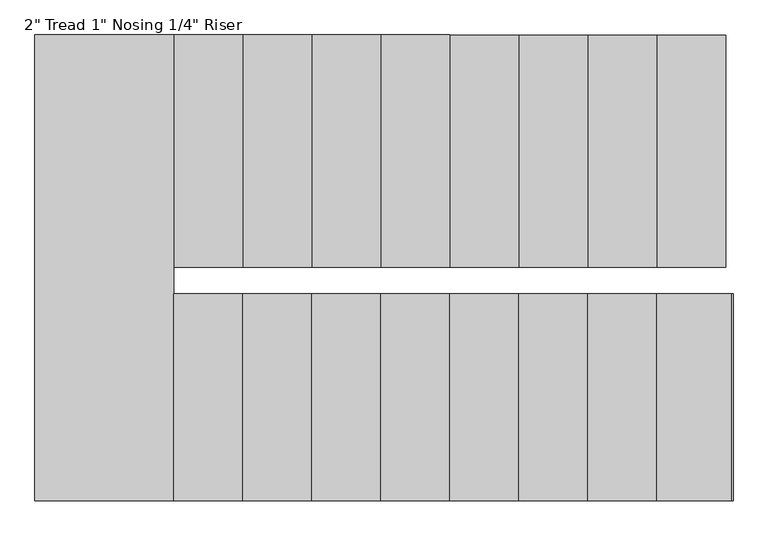
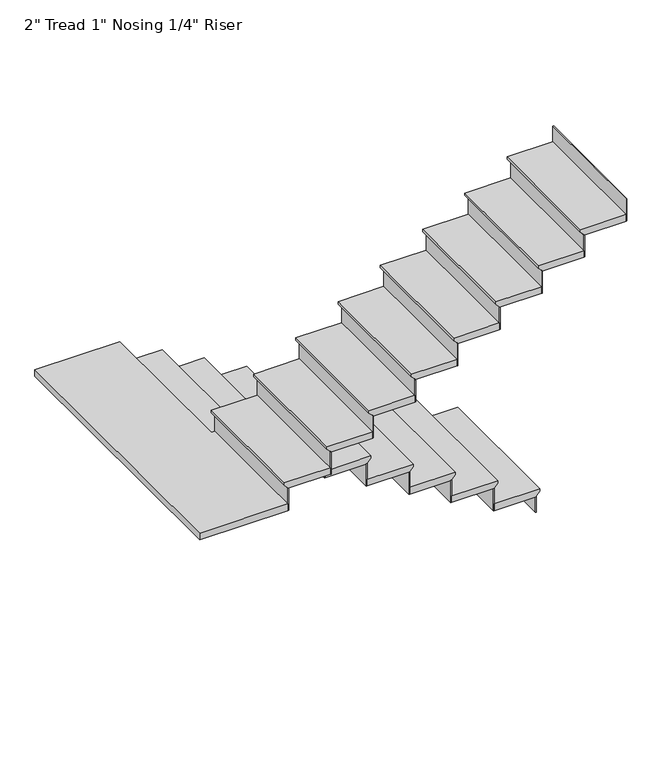
"""IFC4 building model written with IfcOpenShell, lengths in millimetres: stair flight geometry."""

from ifc_helpers import new_model, si_unit, origin, place, context, project, spatial, faceted_brep, source, transform, mapped, element, save


def stair_flight_dc0a5270(model_context):
    return source(origin(), model_context, "Body", "Brep", [
        faceted_brep([(4295.1355783, 9969.5, 150.2833333), (4295.1355783, 9969.5, 169.3333333), (4295.1355783, 8944.6068332, 169.3333333), (4295.1355783, 8944.6068332, 150.2833333), (4269.7355783, 9969.5, 124.8833333), (4269.7355783, 8944.6068332, 124.8833333), (3964.9355783, 9969.5, 169.3333333), (3964.9355783, 8944.6068332, 169.3333333), (4269.7355783, 8944.6068332, 118.5333333), (3964.9355783, 8944.6068332, 118.5333333), (3964.9355783, 9969.5, 118.5333333), (4269.7355783, 9969.5, 118.5333333)], [[[0, 1, 2, 3]], [[4, 0, 3, 5]], [[2, 1, 6, 7]], [[8, 9, 10, 11]], [[2, 7, 9, 8, 5, 3]], [[8, 11, 4, 5]], [[6, 1, 0, 4, 11, 10]], [[7, 6, 10, 9]]]),
        faceted_brep([(4269.7355783, 9969.5, 118.5333333), (4269.7355783, 9969.5, 0.0), (4263.3855783, 9969.5, 0.0), (4263.3855783, 9969.5, 118.5333333), (4269.7355783, 8944.6068332, 118.5333333), (4263.3855783, 8944.6068332, 118.5333333), (4263.3855783, 8944.6068332, 0.0), (4269.7355783, 8944.6068332, 0.0)], [[[0, 1, 2, 3]], [[4, 5, 6, 7]], [[1, 0, 4, 7]], [[2, 1, 7, 6]], [[3, 2, 6, 5]], [[0, 3, 5, 4]]]),
        faceted_brep([(3964.9355783, 9969.5, 287.8666667), (3964.9355783, 9969.5, 118.5333333), (3958.5855783, 9969.5, 118.5333333), (3958.5855783, 9969.5, 287.8666667), (3964.9355783, 8944.6068332, 287.8666667), (3958.5855783, 8944.6068332, 287.8666667), (3958.5855783, 8944.6068332, 118.5333333), (3964.9355783, 8944.6068332, 118.5333333)], [[[0, 1, 2, 3]], [[4, 5, 6, 7]], [[1, 0, 4, 7]], [[2, 1, 7, 6]], [[3, 2, 6, 5]], [[0, 3, 5, 4]]]),
        faceted_brep([(3990.3355783, 8944.6068332, 338.6666667), (3990.3355783, 9969.5, 338.6666667), (3660.1355783, 9969.5, 338.6666667), (3660.1355783, 8944.6068332, 338.6666667), (3964.9355783, 8944.6068332, 287.8666667), (3660.1355783, 8944.6068332, 287.8666667), (3660.1355783, 9969.5, 287.8666667), (3964.9355783, 9969.5, 287.8666667), (3964.9355783, 8944.6068332, 294.2166667), (3990.3355783, 8944.6068332, 319.6166667), (3964.9355783, 9969.5, 294.2166667), (3990.3355783, 9969.5, 319.6166667)], [[[0, 1, 2, 3]], [[4, 5, 6, 7]], [[0, 3, 5, 4, 8, 9]], [[4, 7, 10, 8]], [[2, 1, 11, 10, 7, 6]], [[3, 2, 6, 5]], [[11, 1, 0, 9]], [[10, 11, 9, 8]]]),
        faceted_brep([(3660.1355783, 9969.5, 457.2), (3660.1355783, 9969.5, 287.8666667), (3653.7855783, 9969.5, 287.8666667), (3653.7855783, 9969.5, 457.2), (3660.1355783, 8944.6068332, 457.2), (3653.7855783, 8944.6068332, 457.2), (3653.7855783, 8944.6068332, 287.8666667), (3660.1355783, 8944.6068332, 287.8666667)], [[[0, 1, 2, 3]], [[4, 5, 6, 7]], [[1, 0, 4, 7]], [[2, 1, 7, 6]], [[3, 2, 6, 5]], [[0, 3, 5, 4]]]),
        faceted_brep([(3685.5355783, 8944.6068332, 508.0), (3685.5355783, 9969.5, 508.0), (3355.3355783, 9969.5, 508.0), (3355.3355783, 8944.6068332, 508.0), (3660.1355783, 8944.6068332, 457.2), (3355.3355783, 8944.6068332, 457.2), (3355.3355783, 9969.5, 457.2), (3660.1355783, 9969.5, 457.2), (3660.1355783, 8944.6068332, 463.55), (3685.5355783, 8944.6068332, 488.95), (3660.1355783, 9969.5, 463.55), (3685.5355783, 9969.5, 488.95)], [[[0, 1, 2, 3]], [[4, 5, 6, 7]], [[0, 3, 5, 4, 8, 9]], [[4, 7, 10, 8]], [[2, 1, 11, 10, 7, 6]], [[3, 2, 6, 5]], [[11, 1, 0, 9]], [[10, 11, 9, 8]]]),
        faceted_brep([(3355.3355783, 9969.5, 626.5333333), (3355.3355783, 9969.5, 457.2), (3348.9855783, 9969.5, 457.2), (3348.9855783, 9969.5, 626.5333333), (3355.3355783, 8944.6068332, 626.5333333), (3348.9855783, 8944.6068332, 626.5333333), (3348.9855783, 8944.6068332, 457.2), (3355.3355783, 8944.6068332, 457.2)], [[[0, 1, 2, 3]], [[4, 5, 6, 7]], [[1, 0, 4, 7]], [[2, 1, 7, 6]], [[3, 2, 6, 5]], [[0, 3, 5, 4]]]),
        faceted_brep([(3380.7355783, 8944.6068332, 677.3333333), (3380.7355783, 9969.5, 677.3333333), (3050.5355783, 9969.5, 677.3333333), (3050.5355783, 8944.6068332, 677.3333333), (3355.3355783, 8944.6068332, 626.5333333), (3050.5355783, 8944.6068332, 626.5333333), (3050.5355783, 9969.5, 626.5333333), (3355.3355783, 9969.5, 626.5333333), (3355.3355783, 8944.6068332, 632.8833333), (3380.7355783, 8944.6068332, 658.2833333), (3355.3355783, 9969.5, 632.8833333), (3380.7355783, 9969.5, 658.2833333)], [[[0, 1, 2, 3]], [[4, 5, 6, 7]], [[0, 3, 5, 4, 8, 9]], [[4, 7, 10, 8]], [[2, 1, 11, 10, 7, 6]], [[3, 2, 6, 5]], [[11, 1, 0, 9]], [[10, 11, 9, 8]]]),
        faceted_brep([(3050.5355783, 9969.5, 795.8666667), (3050.5355783, 9969.5, 626.5333333), (3044.1855783, 9969.5, 626.5333333), (3044.1855783, 9969.5, 795.8666667), (3050.5355783, 8944.6068332, 795.8666667), (3044.1855783, 8944.6068332, 795.8666667), (3044.1855783, 8944.6068332, 626.5333333), (3050.5355783, 8944.6068332, 626.5333333)], [[[0, 1, 2, 3]], [[4, 5, 6, 7]], [[1, 0, 4, 7]], [[2, 1, 7, 6]], [[3, 2, 6, 5]], [[0, 3, 5, 4]]]),
        faceted_brep([(3075.9355783, 8944.6068332, 846.6666667), (3075.9355783, 9969.5, 846.6666667), (2745.7355783, 9969.5, 846.6666667), (2745.7355783, 8944.6068332, 846.6666667), (3050.5355783, 8944.6068332, 795.8666667), (2745.7355783, 8944.6068332, 795.8666667), (2745.7355783, 9969.5, 795.8666667), (3050.5355783, 9969.5, 795.8666667), (3050.5355783, 8944.6068332, 802.2166667), (3075.9355783, 8944.6068332, 827.6166667), (3050.5355783, 9969.5, 802.2166667), (3075.9355783, 9969.5, 827.6166667)], [[[0, 1, 2, 3]], [[4, 5, 6, 7]], [[0, 3, 5, 4, 8, 9]], [[4, 7, 10, 8]], [[2, 1, 11, 10, 7, 6]], [[3, 2, 6, 5]], [[11, 1, 0, 9]], [[10, 11, 9, 8]]]),
        faceted_brep([(2745.7355783, 9969.5, 965.2), (2745.7355783, 9969.5, 795.8666667), (2739.3855783, 9969.5, 795.8666667), (2739.3855783, 9969.5, 965.2), (2745.7355783, 8944.6068332, 965.2), (2739.3855783, 8944.6068332, 965.2), (2739.3855783, 8944.6068332, 795.8666667), (2745.7355783, 8944.6068332, 795.8666667)], [[[0, 1, 2, 3]], [[4, 5, 6, 7]], [[1, 0, 4, 7]], [[2, 1, 7, 6]], [[3, 2, 6, 5]], [[0, 3, 5, 4]]]),
        faceted_brep([(2771.1355783, 8944.6068332, 1016.0), (2771.1355783, 9969.5, 1016.0), (2440.9355783, 9969.5, 1016.0), (2440.9355783, 8944.6068332, 1016.0), (2745.7355783, 8944.6068332, 965.2), (2440.9355783, 8944.6068332, 965.2), (2440.9355783, 9969.5, 965.2), (2745.7355783, 9969.5, 965.2), (2745.7355783, 8944.6068332, 971.55), (2771.1355783, 8944.6068332, 996.95), (2745.7355783, 9969.5, 971.55), (2771.1355783, 9969.5, 996.95)], [[[0, 1, 2, 3]], [[4, 5, 6, 7]], [[0, 3, 5, 4, 8, 9]], [[4, 7, 10, 8]], [[2, 1, 11, 10, 7, 6]], [[3, 2, 6, 5]], [[11, 1, 0, 9]], [[10, 11, 9, 8]]]),
        faceted_brep([(2440.9355783, 9969.5, 1134.5333333), (2440.9355783, 9969.5, 965.2), (2434.5855783, 9969.5, 965.2), (2434.5855783, 9969.5, 1134.5333333), (2440.9355783, 8944.6068332, 1134.5333333), (2434.5855783, 8944.6068332, 1134.5333333), (2434.5855783, 8944.6068332, 965.2), (2440.9355783, 8944.6068332, 965.2)], [[[0, 1, 2, 3]], [[4, 5, 6, 7]], [[1, 0, 4, 7]], [[2, 1, 7, 6]], [[3, 2, 6, 5]], [[0, 3, 5, 4]]]),
        faceted_brep([(2466.3355783, 8944.6068332, 1185.3333333), (2466.3355783, 9969.5, 1185.3333333), (2136.1355783, 9969.5, 1185.3333333), (2136.1355783, 8944.6068332, 1185.3333333), (2440.9355783, 8944.6068332, 1134.5333333), (2136.1355783, 8944.6068332, 1134.5333333), (2136.1355783, 9969.5, 1134.5333333), (2440.9355783, 9969.5, 1134.5333333), (2440.9355783, 8944.6068332, 1140.8833333), (2466.3355783, 8944.6068332, 1166.2833333), (2440.9355783, 9969.5, 1140.8833333), (2466.3355783, 9969.5, 1166.2833333)], [[[0, 1, 2, 3]], [[4, 5, 6, 7]], [[0, 3, 5, 4, 8, 9]], [[4, 7, 10, 8]], [[2, 1, 11, 10, 7, 6]], [[3, 2, 6, 5]], [[11, 1, 0, 9]], [[10, 11, 9, 8]]]),
        faceted_brep([(2136.1355783, 9969.5, 1303.8666667), (2136.1355783, 9969.5, 1134.5333333), (2129.7855783, 9969.5, 1134.5333333), (2129.7855783, 9969.5, 1303.8666667), (2136.1355783, 8944.6068332, 1303.8666667), (2129.7855783, 8944.6068332, 1303.8666667), (2129.7855783, 8944.6068332, 1134.5333333), (2136.1355783, 8944.6068332, 1134.5333333)], [[[0, 1, 2, 3]], [[4, 5, 6, 7]], [[1, 0, 4, 7]], [[2, 1, 7, 6]], [[3, 2, 6, 5]], [[0, 3, 5, 4]]]),
        faceted_brep([(2161.5355783, 8944.6068332, 1354.6666667), (2161.5355783, 9969.5, 1354.6666667), (1831.3355783, 9969.5, 1354.6666667), (1831.3355783, 8944.6068332, 1354.6666667), (2136.1355783, 8944.6068332, 1303.8666667), (1831.3355783, 8944.6068332, 1303.8666667), (1831.3355783, 9969.5, 1303.8666667), (2136.1355783, 9969.5, 1303.8666667), (2136.1355783, 8944.6068332, 1310.2166667), (2161.5355783, 8944.6068332, 1335.6166667), (2136.1355783, 9969.5, 1310.2166667), (2161.5355783, 9969.5, 1335.6166667)], [[[0, 1, 2, 3]], [[4, 5, 6, 7]], [[0, 3, 5, 4, 8, 9]], [[4, 7, 10, 8]], [[2, 1, 11, 10, 7, 6]], [[3, 2, 6, 5]], [[11, 1, 0, 9]], [[10, 11, 9, 8]]]),
        faceted_brep([(1831.3355783, 9969.5, 1473.2), (1831.3355783, 9969.5, 1303.8666667), (1824.9855783, 9969.5, 1303.8666667), (1824.9855783, 9969.5, 1473.2), (1831.3355783, 8944.6068332, 1473.2), (1824.9855783, 8944.6068332, 1473.2), (1824.9855783, 8944.6068332, 1303.8666667), (1831.3355783, 8944.6068332, 1303.8666667)], [[[0, 1, 2, 3]], [[4, 5, 6, 7]], [[1, 0, 4, 7]], [[2, 1, 7, 6]], [[3, 2, 6, 5]], [[0, 3, 5, 4]]]),
        faceted_brep([(1882.1355783, 8826.5, 1524.0), (1856.7355783, 8826.5, 1524.0), (1856.7355783, 9969.5, 1524.0), (1244.6, 9969.5, 1524.0), (1244.6, 7912.1, 1524.0), (1882.1355783, 7912.1, 1524.0), (1856.7355783, 8826.5, 1473.2), (1882.1355783, 8826.5, 1473.2), (1882.1355783, 7912.1, 1473.2), (1244.6, 7912.1, 1473.2), (1244.6, 9969.5, 1473.2), (1831.3355783, 9969.5, 1473.2), (1831.3355783, 8944.6068332, 1473.2), (1856.7355783, 8944.6068332, 1473.2), (1856.7355783, 8944.6068332, 1504.95), (1856.7355783, 9969.5, 1504.95), (1831.3355783, 8944.6068332, 1479.55), (1831.3355783, 9969.5, 1479.55)], [[[0, 1, 2, 3, 4, 5]], [[6, 7, 8, 9, 10, 11, 12, 13]], [[1, 0, 7, 6]], [[2, 1, 6, 13, 14, 15]], [[13, 12, 16, 14]], [[12, 11, 17, 16]], [[3, 2, 15, 17, 11, 10]], [[4, 3, 10, 9]], [[5, 4, 9, 8]], [[0, 5, 8, 7]], [[17, 15, 14, 16]]]),
        faceted_brep([(1882.1355783, 7912.1, 1642.5333333), (1882.1355783, 7912.1, 1473.2), (1888.4855783, 7912.1, 1473.2), (1888.4855783, 7912.1, 1642.5333333), (1882.1355783, 8826.5, 1642.5333333), (1888.4855783, 8826.5, 1642.5333333), (1888.4855783, 8826.5, 1473.2), (1882.1355783, 8826.5, 1473.2)], [[[0, 1, 2, 3]], [[4, 5, 6, 7]], [[1, 0, 4, 7]], [[2, 1, 7, 6]], [[3, 2, 6, 5]], [[0, 3, 5, 4]]]),
        faceted_brep([(1856.7355783, 8826.5, 1693.3333333), (1856.7355783, 7912.1, 1693.3333333), (2186.9355783, 7912.1, 1693.3333333), (2186.9355783, 8826.5, 1693.3333333), (1882.1355783, 8826.5, 1642.5333333), (2186.9355783, 8826.5, 1642.5333333), (2186.9355783, 7912.1, 1642.5333333), (1882.1355783, 7912.1, 1642.5333333), (1882.1355783, 8826.5, 1648.8833333), (1856.7355783, 8826.5, 1674.2833333), (1882.1355783, 7912.1, 1648.8833333), (1856.7355783, 7912.1, 1674.2833333)], [[[0, 1, 2, 3]], [[4, 5, 6, 7]], [[0, 3, 5, 4, 8, 9]], [[4, 7, 10, 8]], [[2, 1, 11, 10, 7, 6]], [[3, 2, 6, 5]], [[11, 1, 0, 9]], [[10, 11, 9, 8]]]),
        faceted_brep([(2186.9355783, 7912.1, 1811.8666667), (2186.9355783, 7912.1, 1642.5333333), (2193.2855783, 7912.1, 1642.5333333), (2193.2855783, 7912.1, 1811.8666667), (2186.9355783, 8826.5, 1811.8666667), (2193.2855783, 8826.5, 1811.8666667), (2193.2855783, 8826.5, 1642.5333333), (2186.9355783, 8826.5, 1642.5333333)], [[[0, 1, 2, 3]], [[4, 5, 6, 7]], [[1, 0, 4, 7]], [[2, 1, 7, 6]], [[3, 2, 6, 5]], [[0, 3, 5, 4]]]),
        faceted_brep([(2161.5355783, 8826.5, 1862.6666667), (2161.5355783, 7912.1, 1862.6666667), (2491.7355783, 7912.1, 1862.6666667), (2491.7355783, 8826.5, 1862.6666667), (2186.9355783, 8826.5, 1811.8666667), (2491.7355783, 8826.5, 1811.8666667), (2491.7355783, 7912.1, 1811.8666667), (2186.9355783, 7912.1, 1811.8666667), (2186.9355783, 8826.5, 1818.2166667), (2161.5355783, 8826.5, 1843.6166667), (2186.9355783, 7912.1, 1818.2166667), (2161.5355783, 7912.1, 1843.6166667)], [[[0, 1, 2, 3]], [[4, 5, 6, 7]], [[0, 3, 5, 4, 8, 9]], [[4, 7, 10, 8]], [[2, 1, 11, 10, 7, 6]], [[3, 2, 6, 5]], [[11, 1, 0, 9]], [[10, 11, 9, 8]]]),
        faceted_brep([(2491.7355783, 7912.1, 1981.2), (2491.7355783, 7912.1, 1811.8666667), (2498.0855783, 7912.1, 1811.8666667), (2498.0855783, 7912.1, 1981.2), (2491.7355783, 8826.5, 1981.2), (2498.0855783, 8826.5, 1981.2), (2498.0855783, 8826.5, 1811.8666667), (2491.7355783, 8826.5, 1811.8666667)], [[[0, 1, 2, 3]], [[4, 5, 6, 7]], [[1, 0, 4, 7]], [[2, 1, 7, 6]], [[3, 2, 6, 5]], [[0, 3, 5, 4]]]),
        faceted_brep([(2466.3355783, 8826.5, 2032.0), (2466.3355783, 7912.1, 2032.0), (2796.5355783, 7912.1, 2032.0), (2796.5355783, 8826.5, 2032.0), (2491.7355783, 8826.5, 1981.2), (2796.5355783, 8826.5, 1981.2), (2796.5355783, 7912.1, 1981.2), (2491.7355783, 7912.1, 1981.2), (2491.7355783, 8826.5, 1987.55), (2466.3355783, 8826.5, 2012.95), (2491.7355783, 7912.1, 1987.55), (2466.3355783, 7912.1, 2012.95)], [[[0, 1, 2, 3]], [[4, 5, 6, 7]], [[0, 3, 5, 4, 8, 9]], [[4, 7, 10, 8]], [[2, 1, 11, 10, 7, 6]], [[3, 2, 6, 5]], [[11, 1, 0, 9]], [[10, 11, 9, 8]]]),
        faceted_brep([(2796.5355783, 7912.1, 2150.5333333), (2796.5355783, 7912.1, 1981.2), (2802.8855783, 7912.1, 1981.2), (2802.8855783, 7912.1, 2150.5333333), (2796.5355783, 8826.5, 2150.5333333), (2802.8855783, 8826.5, 2150.5333333), (2802.8855783, 8826.5, 1981.2), (2796.5355783, 8826.5, 1981.2)], [[[0, 1, 2, 3]], [[4, 5, 6, 7]], [[1, 0, 4, 7]], [[2, 1, 7, 6]], [[3, 2, 6, 5]], [[0, 3, 5, 4]]]),
        faceted_brep([(2771.1355783, 8826.5, 2201.3333333), (2771.1355783, 7912.1, 2201.3333333), (3101.3355783, 7912.1, 2201.3333333), (3101.3355783, 8826.5, 2201.3333333), (2796.5355783, 8826.5, 2150.5333333), (3101.3355783, 8826.5, 2150.5333333), (3101.3355783, 7912.1, 2150.5333333), (2796.5355783, 7912.1, 2150.5333333), (2796.5355783, 8826.5, 2156.8833333), (2771.1355783, 8826.5, 2182.2833333), (2796.5355783, 7912.1, 2156.8833333), (2771.1355783, 7912.1, 2182.2833333)], [[[0, 1, 2, 3]], [[4, 5, 6, 7]], [[0, 3, 5, 4, 8, 9]], [[4, 7, 10, 8]], [[2, 1, 11, 10, 7, 6]], [[3, 2, 6, 5]], [[11, 1, 0, 9]], [[10, 11, 9, 8]]]),
        faceted_brep([(3101.3355783, 7912.1, 2319.8666667), (3101.3355783, 7912.1, 2150.5333333), (3107.6855783, 7912.1, 2150.5333333), (3107.6855783, 7912.1, 2319.8666667), (3101.3355783, 8826.5, 2319.8666667), (3107.6855783, 8826.5, 2319.8666667), (3107.6855783, 8826.5, 2150.5333333), (3101.3355783, 8826.5, 2150.5333333)], [[[0, 1, 2, 3]], [[4, 5, 6, 7]], [[1, 0, 4, 7]], [[2, 1, 7, 6]], [[3, 2, 6, 5]], [[0, 3, 5, 4]]]),
        faceted_brep([(3075.9355783, 8826.5, 2370.6666667), (3075.9355783, 7912.1, 2370.6666667), (3406.1355783, 7912.1, 2370.6666667), (3406.1355783, 8826.5, 2370.6666667), (3101.3355783, 8826.5, 2319.8666667), (3406.1355783, 8826.5, 2319.8666667), (3406.1355783, 7912.1, 2319.8666667), (3101.3355783, 7912.1, 2319.8666667), (3101.3355783, 8826.5, 2326.2166667), (3075.9355783, 8826.5, 2351.6166667), (3101.3355783, 7912.1, 2326.2166667), (3075.9355783, 7912.1, 2351.6166667)], [[[0, 1, 2, 3]], [[4, 5, 6, 7]], [[0, 3, 5, 4, 8, 9]], [[4, 7, 10, 8]], [[2, 1, 11, 10, 7, 6]], [[3, 2, 6, 5]], [[11, 1, 0, 9]], [[10, 11, 9, 8]]]),
        faceted_brep([(3406.1355783, 7912.1, 2489.2), (3406.1355783, 7912.1, 2319.8666667), (3412.4855783, 7912.1, 2319.8666667), (3412.4855783, 7912.1, 2489.2), (3406.1355783, 8826.5, 2489.2), (3412.4855783, 8826.5, 2489.2), (3412.4855783, 8826.5, 2319.8666667), (3406.1355783, 8826.5, 2319.8666667)], [[[0, 1, 2, 3]], [[4, 5, 6, 7]], [[1, 0, 4, 7]], [[2, 1, 7, 6]], [[3, 2, 6, 5]], [[0, 3, 5, 4]]]),
        faceted_brep([(3380.7355783, 8826.5, 2540.0), (3380.7355783, 7912.1, 2540.0), (3710.9355783, 7912.1, 2540.0), (3710.9355783, 8826.5, 2540.0), (3406.1355783, 8826.5, 2489.2), (3710.9355783, 8826.5, 2489.2), (3710.9355783, 7912.1, 2489.2), (3406.1355783, 7912.1, 2489.2), (3406.1355783, 8826.5, 2495.55), (3380.7355783, 8826.5, 2520.95), (3406.1355783, 7912.1, 2495.55), (3380.7355783, 7912.1, 2520.95)], [[[0, 1, 2, 3]], [[4, 5, 6, 7]], [[0, 3, 5, 4, 8, 9]], [[4, 7, 10, 8]], [[2, 1, 11, 10, 7, 6]], [[3, 2, 6, 5]], [[11, 1, 0, 9]], [[10, 11, 9, 8]]]),
        faceted_brep([(3710.9355783, 7912.1, 2658.5333333), (3710.9355783, 7912.1, 2489.2), (3717.2855783, 7912.1, 2489.2), (3717.2855783, 7912.1, 2658.5333333), (3710.9355783, 8826.5, 2658.5333333), (3717.2855783, 8826.5, 2658.5333333), (3717.2855783, 8826.5, 2489.2), (3710.9355783, 8826.5, 2489.2)], [[[0, 1, 2, 3]], [[4, 5, 6, 7]], [[1, 0, 4, 7]], [[2, 1, 7, 6]], [[3, 2, 6, 5]], [[0, 3, 5, 4]]]),
        faceted_brep([(3685.5355783, 8826.5, 2709.3333333), (3685.5355783, 7912.1, 2709.3333333), (4015.7355783, 7912.1, 2709.3333333), (4015.7355783, 8826.5, 2709.3333333), (3710.9355783, 8826.5, 2658.5333333), (4015.7355783, 8826.5, 2658.5333333), (4015.7355783, 7912.1, 2658.5333333), (3710.9355783, 7912.1, 2658.5333333), (3710.9355783, 8826.5, 2664.8833333), (3685.5355783, 8826.5, 2690.2833333), (3710.9355783, 7912.1, 2664.8833333), (3685.5355783, 7912.1, 2690.2833333)], [[[0, 1, 2, 3]], [[4, 5, 6, 7]], [[0, 3, 5, 4, 8, 9]], [[4, 7, 10, 8]], [[2, 1, 11, 10, 7, 6]], [[3, 2, 6, 5]], [[11, 1, 0, 9]], [[10, 11, 9, 8]]]),
        faceted_brep([(4015.7355783, 7912.1, 2827.8666667), (4015.7355783, 7912.1, 2658.5333333), (4022.0855783, 7912.1, 2658.5333333), (4022.0855783, 7912.1, 2827.8666667), (4015.7355783, 8826.5, 2827.8666667), (4022.0855783, 8826.5, 2827.8666667), (4022.0855783, 8826.5, 2658.5333333), (4015.7355783, 8826.5, 2658.5333333)], [[[0, 1, 2, 3]], [[4, 5, 6, 7]], [[1, 0, 4, 7]], [[2, 1, 7, 6]], [[3, 2, 6, 5]], [[0, 3, 5, 4]]]),
        faceted_brep([(4320.5355783, 7912.1, 2997.2), (4320.5355783, 7912.1, 2827.8666667), (4326.8855783, 7912.1, 2827.8666667), (4326.8855783, 7912.1, 2997.2), (4320.5355783, 8826.5, 2997.2), (4326.8855783, 8826.5, 2997.2), (4326.8855783, 8826.5, 2827.8666667), (4320.5355783, 8826.5, 2827.8666667)], [[[0, 1, 2, 3]], [[4, 5, 6, 7]], [[1, 0, 4, 7]], [[2, 1, 7, 6]], [[3, 2, 6, 5]], [[0, 3, 5, 4]]]),
        faceted_brep([(3990.3355783, 8826.5, 2878.6666667), (3990.3355783, 7912.1, 2878.6666667), (4320.5355783, 7912.1, 2878.6666667), (4320.5355783, 8826.5, 2878.6666667), (4015.7355783, 8826.5, 2827.8666667), (4320.5355783, 8826.5, 2827.8666667), (4320.5355783, 7912.1, 2827.8666667), (4015.7355783, 7912.1, 2827.8666667), (4015.7355783, 8826.5, 2834.2166667), (3990.3355783, 8826.5, 2859.6166667), (4015.7355783, 7912.1, 2834.2166667), (3990.3355783, 7912.1, 2859.6166667)], [[[0, 1, 2, 3]], [[4, 5, 6, 7]], [[0, 3, 5, 4, 8, 9]], [[4, 7, 10, 8]], [[2, 1, 11, 10, 7, 6]], [[3, 2, 6, 5]], [[11, 1, 0, 9]], [[10, 11, 9, 8]]]),
    ])


if __name__ == "__main__":
    model = new_model("IFC4")
    model_context = context("Model", 3, world=origin())
    ifc_project = project(units=[si_unit("LENGTHUNIT", "METRE", prefix="MILLI")], contexts=[model_context])
    site = spatial("IfcSite", under=ifc_project)
    building = spatial("IfcBuilding", under=site)
    placement = place(None, origin())
    stair_flight_shape = stair_flight_dc0a5270(model_context)
    element("IfcStairFlight", 1, ObjectType="2\" Tread 1\" Nosing 1/4\" Riser", at=placement, inside=building, context=model_context, shape_type="MappedRepresentation", body=[
        mapped(stair_flight_shape, transform((0.0, 0.0, 0.0), x_axis=(1.0, 0.0, 0.0), y_axis=(0.0, 1.0, 0.0), z_axis=(0.0, 0.0, 1.0))),
    ])
    save(model, "model.ifc")
